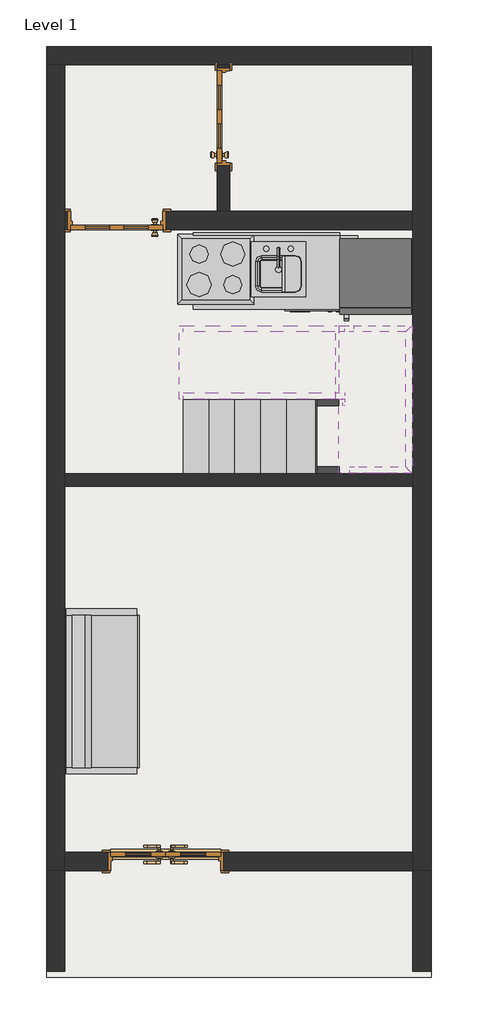
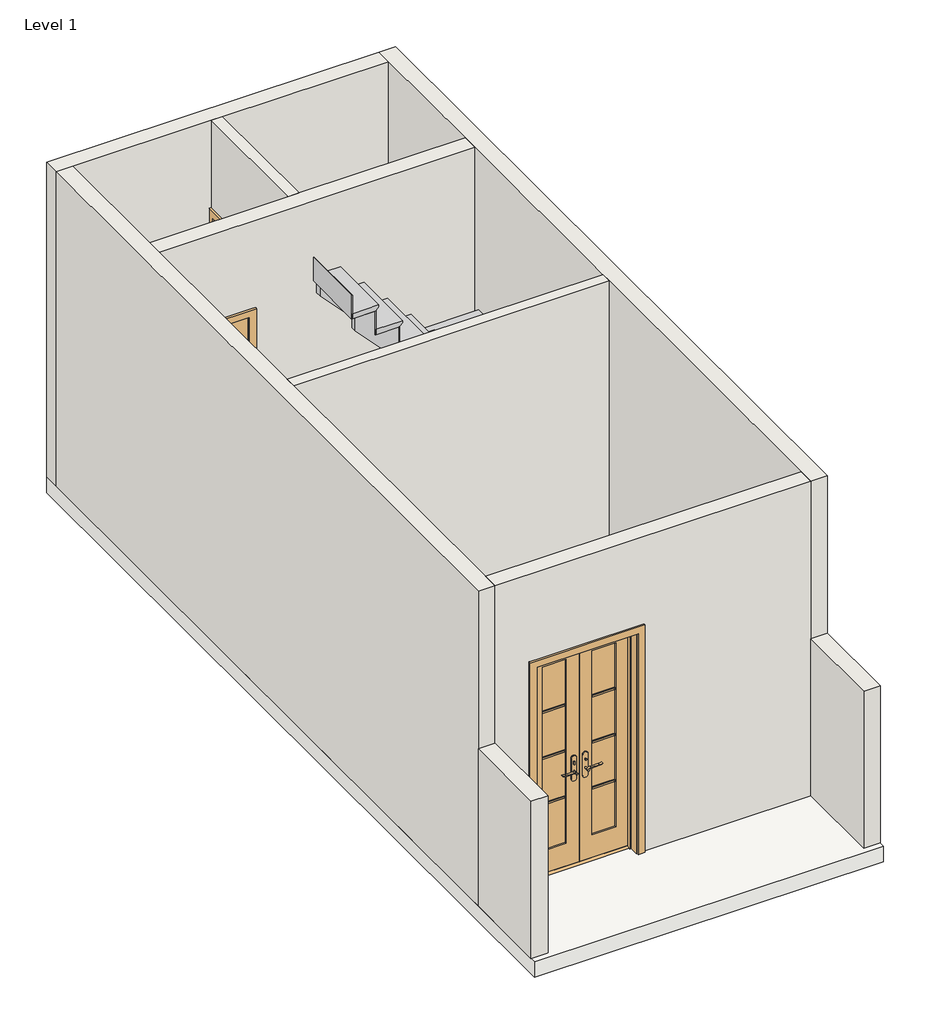
# One storey, incomplete: 9 walls, 8 members, 4 proxies, 3 doors, 2 furniture elements, 2 slabs, 2 stair flights, 1 flow terminal.
"""IFC4 building model written with IfcOpenShell, lengths in millimetres."""

from ifc_helpers import new_model, si_unit, frame, origin, origin_with_axes, place, context, project, spatial, polyline, outline, extrude, faceted_brep, transform, mapped, element, save
from components import proxy_a6faaae8, proxy_45b28599, kitchenette_medium_kitchenette_medium_5bfe328f, proxy_e2b28e2e, door_665efd91, door_a7370db0, door_bd7b73b2, flow_terminal_871c2e40, furniture_a1a13893, furniture_de36dbc2, non_monolithic_landing_e6237f85, stair_flight_15f1c366, stair_flight_6b27b35d

model = new_model("IFC4")

# Units and contexts
model_context = context("Model", 3, world=origin())
ifc_project = project(units=[si_unit("LENGTHUNIT", "METRE", prefix="MILLI")], contexts=[model_context])

# Site, building, storey
site = spatial("IfcSite", under=ifc_project)
building = spatial("IfcBuilding", under=site)
storey = spatial("IfcBuildingStorey", under=building, Name="Level 1", Elevation=0.0)

# Proxies
placement = place(None, origin())
proxy_shape = proxy_a6faaae8(model_context)
element("IfcBuildingElementProxy", 1, Name="Cook Top-4 Unit2 : 22\" x 20\"", ObjectType="Cook Top-4 Unit2 : 22\" x 20\"", at=placement, inside=storey, context=model_context, shape_type="MappedRepresentation", body=[
    mapped(proxy_shape, transform((-4318.156559, 5420.3980625, 0.0), x_axis=(1.0, 0.0, 0.0), y_axis=(0.0, 1.0, 0.0), z_axis=(0.0, 0.0, 1.0))),
])
proxy_2_shape = proxy_45b28599(model_context)
element("IfcBuildingElementProxy", 2, Name="Dishwasher : 24\" x 24\" x 34\"", ObjectType="Dishwasher : 24\" x 24\" x 34\"", at=placement, inside=storey, context=model_context, shape_type="MappedRepresentation", body=[
    mapped(proxy_2_shape, transform((-3824.1740275, 5128.5484977, 0.0), x_axis=(1.0, 0.0, 0.0), y_axis=(0.0, 1.0, 0.0), z_axis=(0.0, 0.0, 1.0))),
])
kitchenette_medium_kitchenette_medium_shape = kitchenette_medium_kitchenette_medium_5bfe328f(model_context)
element("IfcBuildingElementProxy", 3, Name="Kitchenette - Medium : Kitchenette - Medium", ObjectType="Kitchenette - Medium : Kitchenette - Medium", at=placement, inside=storey, context=model_context, shape_type="MappedRepresentation", body=[
    mapped(kitchenette_medium_kitchenette_medium_shape, transform((-4146.3942639, 5725.1980625, 0.0), x_axis=(1.0, 0.0, 0.0), y_axis=(0.0, 1.0, 0.0), z_axis=(0.0, 0.0, 1.0))),
])
proxy_3_shape = proxy_e2b28e2e(model_context)
element("IfcBuildingElementProxy", 4, Name="Refrigerator : 24\" x 25\" LH", ObjectType="Refrigerator : 24\" x 25\" LH", at=placement, inside=storey, context=model_context, shape_type="MappedRepresentation", body=[
    mapped(proxy_3_shape, transform((-2991.006559, 5374.749091, 0.0), x_axis=(1.0, 0.0, 0.0), y_axis=(0.0, 1.0, 0.0), z_axis=(0.0, 0.0, 1.0))),
])

# Doors
door_shape = door_665efd91(model_context)
element("IfcDoor", 5, ObjectType="Door-Exterior-Double-Full Glass-Wood_Clad : 36\" x 84\"", at=placement, inside=storey, context=model_context, shape_type="MappedRepresentation", body=[
    mapped(door_shape, transform((-4737.256559, 495.9730625, 0.0), x_axis=(1.0, 0.0, 0.0), y_axis=(0.0, 1.0, 0.0), z_axis=(0.0, 0.0, 1.0))),
])
door_2_shape = door_a7370db0(model_context)
element("IfcDoor", 6, ObjectType="Door-Interior-Single-4_Panel-Wood : 30\" x 84\"", at=placement, inside=storey, context=model_context, shape_type="MappedRepresentation", body=[
    mapped(door_2_shape, transform((-5143.656559, 5823.6230625, 0.0), x_axis=(-1.0, 0.0, 0.0), y_axis=(0.0, -1.0, 0.0), z_axis=(0.0, 0.0, 1.0))),
])
door_3_shape = door_bd7b73b2(model_context)
element("IfcDoor", 7, ObjectType="Door-Interior-Single-4_Panel-Wood : 30\" x 84\"", at=placement, inside=storey, context=model_context, shape_type="MappedRepresentation", body=[
    mapped(door_3_shape, transform((-4257.831559, 6690.3980625, 0.0), x_axis=(0.0, 1.0, 0.0), y_axis=(-1.0, 0.0, 0.0), z_axis=(0.0, 0.0, 1.0))),
])

# Flow terminal
flow_terminal_shape = flow_terminal_871c2e40(model_context)
element("IfcFlowTerminal", 8, ObjectType="Sink Kitchen-Island : 18\" x 18\"", at=placement, inside=storey, context=model_context, shape_type="MappedRepresentation", body=[
    mapped(flow_terminal_shape, transform((-3813.1457996, 5418.0526614, -14.4), x_axis=(1.0, 0.0, 0.0), y_axis=(0.0, 1.0, 0.0), z_axis=(0.0, 0.0, 1.0))),
])

# Furniture
furniture_shape = furniture_a1a13893(model_context)
element("IfcFurniture", 9, ObjectType="Counter Top w Sink Hole : 24\" Depth", at=placement, inside=storey, context=model_context, shape_type="MappedRepresentation", body=[
    mapped(furniture_shape, transform((-3308.1942639, 5725.1980625, -14.4), x_axis=(1.0, 0.0, 0.0), y_axis=(0.0, 1.0, 0.0), z_axis=(0.0, 0.0, 1.0))),
])
furniture_2_shape = furniture_de36dbc2(model_context)
element("IfcFurniture", 10, ObjectType="Sofa : 54\"", at=placement, inside=storey, context=model_context, shape_type="MappedRepresentation", body=[
    mapped(furniture_2_shape, transform((-5086.4024607, 1838.4775707, 0.0), x_axis=(0.0, 1.0000000000000002, 0.0), y_axis=(-1.0000000000000002, 0.0, 0.0), z_axis=(0.0, 0.0, 1.0))),
])

# Members
element("IfcMember", 11, ObjectType="Carriage - 2\" Width", at=placement, inside=storey, context=model_context, shape_type="Brep", body=[
    faceted_brep([(-3327.7737097, 4341.1083475, 1778.0), (-3327.7737097, 4391.9083475, 1778.0), (-3543.6737097, 4391.9083475, 1778.0), (-3543.6737097, 4341.1083475, 1778.0), (-3327.7737097, 4341.1083475, 1549.4), (-3327.7737097, 4391.9083475, 1549.4), (-3543.6737097, 4341.1083475, 2006.6), (-3543.6737097, 4391.9083475, 2006.6), (-3759.5737097, 4391.9083475, 2006.6), (-3759.5737097, 4341.1083475, 2006.6), (-3759.5737097, 4341.1083475, 2235.2), (-3759.5737097, 4391.9083475, 2235.2), (-3975.4737097, 4391.9083475, 2235.2), (-3975.4737097, 4341.1083475, 2235.2), (-3975.4737097, 4341.1083475, 2463.8), (-3975.4737097, 4391.9083475, 2463.8), (-4191.3737097, 4391.9083475, 2463.8), (-4191.3737097, 4341.1083475, 2463.8), (-4191.3737097, 4341.1083475, 2692.4), (-4191.3737097, 4391.9083475, 2692.4), (-4407.2737097, 4391.9083475, 2692.4), (-4407.2737097, 4341.1083475, 2692.4), (-4407.2737097, 4341.1083475, 2921.0), (-4407.2737097, 4391.9083475, 2921.0), (-4591.4237097, 4391.9083475, 2921.0), (-4591.4237097, 4341.1083475, 2921.0), (-3245.2237097, 4341.1083475, 1371.6), (-3245.2237097, 4391.9083475, 1371.6), (-3245.2237097, 4391.9083475, 1549.4), (-3245.2237097, 4341.1083475, 1549.4), (-3247.1951617, 4341.1083475, 1371.6), (-3247.1951617, 4391.9083475, 1371.6), (-4591.4237097, 4391.9083475, 2794.9008155), (-4591.4237097, 4341.1083475, 2794.9008155), (-3296.0237097, 4341.1083475, 1423.3008155), (-3327.7737097, 4341.1083475, 1456.9184625), (-3543.6737097, 4341.1083475, 1685.5184625), (-3759.5737097, 4341.1083475, 1914.1184625), (-3975.4737097, 4341.1083475, 2142.7184625), (-4191.3737097, 4341.1083475, 2371.3184625), (-4407.2737097, 4341.1083475, 2599.9184625), (-3296.0237097, 4341.1083475, 1549.4)], [[[0, 1, 2, 3]], [[1, 0, 4, 5]], [[6, 7, 8, 9]], [[3, 2, 7, 6]], [[10, 11, 12, 13]], [[9, 8, 11, 10]], [[14, 15, 16, 17]], [[13, 12, 15, 14]], [[18, 19, 20, 21]], [[17, 16, 19, 18]], [[22, 23, 24, 25]], [[21, 20, 23, 22]], [[26, 27, 28, 29]], [[26, 30, 31, 27]], [[32, 33, 25, 24]], [[31, 32, 24, 23, 20, 19, 16, 15, 12, 11, 8, 7, 2, 1, 5, 28, 27]], [[33, 32, 31, 30, 34, 35, 36, 37, 38, 39, 40]], [[30, 26, 29, 41, 4, 0, 3, 6, 9, 10, 13, 14, 17, 18, 21, 22, 25, 33, 40, 39, 38, 37, 36, 35, 34]], [[5, 4, 41, 29, 28]]]),
])
element("IfcMember", 12, ObjectType="Carriage - 2\" Width", at=placement, inside=storey, context=model_context, shape_type="Brep", body=[
    faceted_brep([(-4591.4237097, 4950.7083475, 2794.9008155), (-4591.4237097, 4899.9083475, 2794.9008155), (-4591.4237097, 4899.9083475, 2921.0), (-4591.4237097, 4950.7083475, 2921.0), (-3247.1951617, 4899.9083475, 1371.6), (-3170.555096, 4899.9083475, 1549.4), (-3327.7737097, 4899.9083475, 1549.4), (-3327.7737097, 4899.9083475, 1778.0), (-3543.6737097, 4899.9083475, 1778.0), (-3543.6737097, 4899.9083475, 2006.6), (-3759.5737097, 4899.9083475, 2006.6), (-3759.5737097, 4899.9083475, 2235.2), (-3975.4737097, 4899.9083475, 2235.2), (-3975.4737097, 4899.9083475, 2463.8), (-4191.3737097, 4899.9083475, 2463.8), (-4191.3737097, 4899.9083475, 2692.4), (-4407.2737097, 4899.9083475, 2692.4), (-4407.2737097, 4899.9083475, 2921.0), (-4407.2737097, 4950.7083475, 2599.9184625), (-4191.3737097, 4950.7083475, 2371.3184625), (-3975.4737097, 4950.7083475, 2142.7184625), (-3759.5737097, 4950.7083475, 1914.1184625), (-3543.6737097, 4950.7083475, 1685.5184625), (-3327.7737097, 4950.7083475, 1456.9184625), (-3296.0237097, 4950.7083475, 1423.3008155), (-3247.1951617, 4950.7083475, 1371.6), (-4407.2737097, 4950.7083475, 2921.0), (-4407.2737097, 4950.7083475, 2692.4), (-4191.3737097, 4950.7083475, 2692.4), (-4191.3737097, 4950.7083475, 2463.8), (-3975.4737097, 4950.7083475, 2463.8), (-3975.4737097, 4950.7083475, 2235.2), (-3759.5737097, 4950.7083475, 2235.2), (-3759.5737097, 4950.7083475, 2006.6), (-3543.6737097, 4950.7083475, 2006.6), (-3543.6737097, 4950.7083475, 1778.0), (-3327.7737097, 4950.7083475, 1778.0), (-3327.7737097, 4950.7083475, 1549.4), (-3296.0237097, 4950.7083475, 1549.4), (-3170.555096, 4950.7083475, 1549.4)], [[[0, 1, 2, 3]], [[1, 4, 5, 6, 7, 8, 9, 10, 11, 12, 13, 14, 15, 16, 17, 2]], [[1, 0, 18, 19, 20, 21, 22, 23, 24, 25, 4]], [[0, 3, 26, 27, 28, 29, 30, 31, 32, 33, 34, 35, 36, 37, 38, 39, 25, 24, 23, 22, 21, 20, 19, 18]], [[7, 36, 35, 8]], [[36, 7, 6, 37]], [[9, 34, 33, 10]], [[8, 35, 34, 9]], [[11, 32, 31, 12]], [[10, 33, 32, 11]], [[13, 30, 29, 14]], [[12, 31, 30, 13]], [[15, 28, 27, 16]], [[14, 29, 28, 15]], [[17, 26, 3, 2]], [[16, 27, 26, 17]], [[4, 25, 39, 5]], [[37, 6, 5, 39, 38]]]),
])
element("IfcMember", 13, ObjectType="Carriage - 2\" Width", at=placement, inside=storey, context=model_context, shape_type="Brep", body=[
    faceted_brep([(-4559.6737097, 4334.5480625, 0.0), (-4424.3522576, 4334.5480625, 0.0), (-4424.3522576, 4283.7480625, 0.0), (-4559.6737097, 4283.7480625, 0.0), (-3296.0237097, 4334.5480625, 1194.7008155), (-3296.0237097, 4283.7480625, 1194.7008155), (-4343.7737097, 4334.5480625, 85.3184625), (-4127.8737097, 4334.5480625, 313.9184625), (-3911.9737097, 4334.5480625, 542.5184625), (-3696.0737097, 4334.5480625, 771.1184625), (-3480.1737097, 4334.5480625, 999.7184625), (-3296.0237097, 4334.5480625, 1320.8), (-4559.6737097, 4334.5480625, 177.8), (-4343.7737097, 4334.5480625, 177.8), (-4343.7737097, 4334.5480625, 406.4), (-4127.8737097, 4334.5480625, 406.4), (-4127.8737097, 4334.5480625, 635.0), (-3911.9737097, 4334.5480625, 635.0), (-3911.9737097, 4334.5480625, 863.6), (-3696.0737097, 4334.5480625, 863.6), (-3696.0737097, 4334.5480625, 1092.2), (-3480.1737097, 4334.5480625, 1092.2), (-3480.1737097, 4334.5480625, 1320.8), (-3480.1737097, 4283.7480625, 1320.8), (-3296.0237097, 4283.7480625, 1320.8), (-3480.1737097, 4283.7480625, 1092.2), (-3696.0737097, 4283.7480625, 1092.2), (-3696.0737097, 4283.7480625, 863.6), (-3911.9737097, 4283.7480625, 863.6), (-3911.9737097, 4283.7480625, 635.0), (-4127.8737097, 4283.7480625, 635.0), (-4127.8737097, 4283.7480625, 406.4), (-4343.7737097, 4283.7480625, 406.4), (-4343.7737097, 4283.7480625, 177.8), (-4559.6737097, 4283.7480625, 177.8)], [[[0, 1, 2, 3]], [[4, 5, 2, 1, 6, 7, 8, 9, 10]], [[11, 4, 10, 9, 8, 7, 6, 1, 0, 12, 13, 14, 15, 16, 17, 18, 19, 20, 21, 22]], [[22, 23, 24, 11]], [[2, 5, 24, 23, 25, 26, 27, 28, 29, 30, 31, 32, 33, 34, 3]], [[34, 12, 0, 3]], [[12, 34, 33, 13]], [[13, 33, 32, 14]], [[14, 32, 31, 15]], [[15, 31, 30, 16]], [[16, 30, 29, 17]], [[17, 29, 28, 18]], [[18, 28, 27, 19]], [[19, 27, 26, 20]], [[20, 26, 25, 21]], [[21, 25, 23, 22]], [[5, 4, 11, 24]]]),
])
element("IfcMember", 14, ObjectType="Carriage - 2\" Width", at=placement, inside=storey, context=model_context, shape_type="Brep", body=[
    faceted_brep([(-4559.6737097, 3775.7480625, 0.0), (-4424.3522576, 3775.7480625, 0.0), (-4424.3522576, 3724.9480625, 0.0), (-4559.6737097, 3724.9480625, 0.0), (-3128.9522576, 3775.7480625, 1371.6), (-3128.9522576, 3724.9480625, 1371.6), (-3264.2737097, 3724.9480625, 1228.3184625), (-3296.0237097, 3724.9480625, 1194.7008155), (-3480.1737097, 3724.9480625, 999.7184625), (-3696.0737097, 3724.9480625, 771.1184625), (-3911.9737097, 3724.9480625, 542.5184625), (-4127.8737097, 3724.9480625, 313.9184625), (-4343.7737097, 3724.9480625, 85.3184625), (-3205.5923234, 3775.7480625, 1549.4), (-4559.6737097, 3775.7480625, 177.8), (-4343.7737097, 3775.7480625, 177.8), (-4343.7737097, 3775.7480625, 406.4), (-4127.8737097, 3775.7480625, 406.4), (-4127.8737097, 3775.7480625, 635.0), (-3911.9737097, 3775.7480625, 635.0), (-3911.9737097, 3775.7480625, 863.6), (-3696.0737097, 3775.7480625, 863.6), (-3696.0737097, 3775.7480625, 1092.2), (-3480.1737097, 3775.7480625, 1092.2), (-3480.1737097, 3775.7480625, 1320.8), (-3264.2737097, 3775.7480625, 1320.8), (-3264.2737097, 3775.7480625, 1549.4), (-3480.1737097, 3724.9480625, 1320.8), (-3296.0237097, 3724.9480625, 1320.8), (-3264.2737097, 3724.9480625, 1320.8), (-3205.5923234, 3724.9480625, 1549.4), (-3264.2737097, 3724.9480625, 1549.4), (-3480.1737097, 3724.9480625, 1092.2), (-3696.0737097, 3724.9480625, 1092.2), (-3696.0737097, 3724.9480625, 863.6), (-3911.9737097, 3724.9480625, 863.6), (-3911.9737097, 3724.9480625, 635.0), (-4127.8737097, 3724.9480625, 635.0), (-4127.8737097, 3724.9480625, 406.4), (-4343.7737097, 3724.9480625, 406.4), (-4343.7737097, 3724.9480625, 177.8), (-4559.6737097, 3724.9480625, 177.8)], [[[0, 1, 2, 3]], [[4, 5, 6, 7, 8, 9, 10, 11, 12, 2, 1]], [[13, 4, 1, 0, 14, 15, 16, 17, 18, 19, 20, 21, 22, 23, 24, 25, 26]], [[24, 27, 28, 29, 25]], [[5, 30, 31, 29, 28, 27, 32, 33, 34, 35, 36, 37, 38, 39, 40, 41, 3, 2, 12, 11, 10, 9, 8, 7, 6]], [[41, 14, 0, 3]], [[14, 41, 40, 15]], [[15, 40, 39, 16]], [[16, 39, 38, 17]], [[17, 38, 37, 18]], [[18, 37, 36, 19]], [[19, 36, 35, 20]], [[20, 35, 34, 21]], [[21, 34, 33, 22]], [[22, 33, 32, 23]], [[23, 32, 27, 24]], [[5, 4, 13, 30]], [[25, 29, 31, 26]], [[26, 31, 30, 13]]]),
])
element("IfcMember", 15, ObjectType="Carriage - 2\" Width", at=placement, inside=storey, context=model_context, shape_type="SweptSolid", body=[
    extrude(outline(polyline([(-3245.2237097, 4341.1083475), (-3245.2237097, 4283.7480625), (-3264.2737097, 4283.7480625), (-3264.2737097, 4334.5480625), (-3296.0237097, 4334.5480625), (-3296.0237097, 4341.1083475), (-3245.2237097, 4341.1083475)])), frame((0.0, 0.0, 1371.6), z_axis=(0.0, 0.0, 1.0), x_axis=(1.0, 0.0, 0.0)), (0.0, 0.0, 1.0), 177.8),
])
element("IfcMember", 16, ObjectType="Carriage - 2\" Width", at=placement, inside=storey, context=model_context, shape_type="Brep", body=[
    faceted_brep([(-2737.2237097, 3775.7480625, 1371.6), (-3128.9522576, 3775.7480625, 1371.6), (-3205.5923234, 3775.7480625, 1549.4), (-2737.2237097, 3775.7480625, 1549.4), (-2686.4237097, 3724.9480625, 1371.6), (-3128.9522576, 3724.9480625, 1371.6), (-2686.4237097, 3724.9480625, 1549.4), (-3205.5923234, 3724.9480625, 1549.4)], [[[0, 1, 2, 3]], [[1, 0, 4, 5]], [[5, 4, 6, 7]], [[3, 2, 7, 6]], [[1, 5, 7, 2]], [[4, 0, 3, 6]]]),
])
element("IfcMember", 17, ObjectType="Carriage - 2\" Width", at=placement, inside=storey, context=model_context, shape_type="SweptSolid", body=[
    extrude(outline(polyline([(-2737.2237097, 3775.7480625), (-2737.2237097, 4899.9083475), (-2686.4237097, 4950.7083475), (-2686.4237097, 3724.9480625), (-2737.2237097, 3775.7480625)])), frame((0.0, 0.0, 1371.6), z_axis=(0.0, 0.0, 1.0), x_axis=(1.0, 0.0, 0.0)), (0.0, 0.0, 1.0), 177.8),
])
element("IfcMember", 18, ObjectType="Carriage - 2\" Width", at=placement, inside=storey, context=model_context, shape_type="Brep", body=[
    faceted_brep([(-3247.1951617, 4899.9083475, 1371.6), (-2737.2237097, 4899.9083475, 1371.6), (-2737.2237097, 4899.9083475, 1549.4), (-3170.555096, 4899.9083475, 1549.4), (-3247.1951617, 4950.7083475, 1371.6), (-2686.4237097, 4950.7083475, 1371.6), (-3170.555096, 4950.7083475, 1549.4), (-2686.4237097, 4950.7083475, 1549.4)], [[[0, 1, 2, 3]], [[1, 0, 4, 5]], [[5, 4, 6, 7]], [[3, 2, 7, 6]], [[1, 5, 7, 2]], [[4, 0, 3, 6]]]),
])

# Slabs
element("IfcSlab", 19, ObjectType="6\"", at=placement, inside=storey, context=model_context, shape_type="SweptSolid", body=[
    extrude(outline(polyline([(-2527.456559, 7274.5980625), (-2527.456559, -472.4019375), (-5727.856559, -472.4019375), (-5727.856559, 7274.5980625), (-2527.456559, 7274.5980625)])), frame((0.0, 0.0, -152.4), z_axis=(0.0, 0.0, 1.0), x_axis=(1.0, 0.0, 0.0)), (0.0, 0.0, 1.0), 152.4),
])
non_monolithic_landing_shape = non_monolithic_landing_e6237f85(model_context)
element("IfcSlab", 20, ObjectType="Non-Monolithic Landing", at=placement, inside=storey, context=model_context, shape_type="MappedRepresentation", body=[
    mapped(non_monolithic_landing_shape, transform((0.0, 0.0, 0.0), x_axis=(1.0, 0.0, 0.0), y_axis=(0.0, 1.0, 0.0), z_axis=(0.0, 0.0, 1.0))),
])

# Stair flights
stair_flight_shape = stair_flight_15f1c366(model_context)
element("IfcStairFlight", 21, ObjectType="2\" Tread 1\" Nosing 1/4\" Riser", at=placement, inside=storey, context=model_context, shape_type="MappedRepresentation", body=[
    mapped(stair_flight_shape, transform((0.0, 0.0, 0.0), x_axis=(1.0, 0.0, 0.0), y_axis=(0.0, 1.0, 0.0), z_axis=(0.0, 0.0, 1.0))),
])
stair_flight_2_shape = stair_flight_6b27b35d(model_context)
element("IfcStairFlight", 22, ObjectType="2\" Tread 1\" Nosing 1/4\" Riser", at=placement, inside=storey, context=model_context, shape_type="MappedRepresentation", body=[
    mapped(stair_flight_2_shape, transform((0.0, 0.0, 0.0), x_axis=(1.0, 0.0, 0.0), y_axis=(0.0, 1.0, 0.0), z_axis=(0.0, 0.0, 1.0))),
])

# Walls
element("IfcWall", 23, ObjectType="4\"", at=placement, inside=storey, context=model_context, shape_type="SweptSolid", body=[
    extrude(outline(polyline([(5902.9980625, 3048.0), (7122.1980625, 3048.0), (7122.1980625, 0.0), (7096.7980625, 0.0), (7096.7980625, 2159.0), (6283.9980625, 2159.0), (6283.9980625, 0.0), (5902.9980625, 0.0), (5902.9980625, 3048.0)])), frame((-4305.456559, 0.0, 0.0), z_axis=(1.0, 0.0, 0.0), x_axis=(0.0, 1.0, 0.0)), (0.0, 0.0, 1.0), 101.6),
])
element("IfcWall", 24, ObjectType="4\"", at=placement, inside=storey, context=model_context, shape_type="SweptSolid", body=[
    extrude(outline(polyline([(-5575.456559, 3718.5980625), (-2679.856559, 3718.5980625), (-2679.856559, 3616.9980625), (-5575.456559, 3616.9980625), (-5575.456559, 3718.5980625)])), origin_with_axes(), (0.0, 0.0, 1.0), 3048.0),
])
element("IfcWall", 25, ObjectType="6\"", at=placement, inside=storey, context=model_context, shape_type="Brep", body=[
    faceted_brep([(-5727.856559, 7122.1980625, 0.0), (-5575.456559, 7122.1980625, 0.0), (-4305.456559, 7122.1980625, 0.0), (-4203.856559, 7122.1980625, 0.0), (-2679.856559, 7122.1980625, 0.0), (-2679.856559, 7122.1980625, 3048.0), (-4203.856559, 7122.1980625, 3048.0), (-4305.456559, 7122.1980625, 3048.0), (-5575.456559, 7122.1980625, 3048.0), (-5727.856559, 7122.1980625, 3048.0), (-5727.856559, 7274.5980625, 0.0), (-5727.856559, 7274.5980625, 3048.0), (-2679.856559, 7274.5980625, 3048.0), (-2679.856559, 7274.5980625, 0.0)], [[[0, 1, 2, 3, 4, 5, 6, 7, 8, 9]], [[10, 11, 12, 13]], [[4, 3, 2, 1, 0, 10, 13]], [[9, 8, 7, 6, 5, 12, 11]], [[0, 9, 11, 10]], [[5, 4, 13, 12]]]),
])
element("IfcWall", 26, ObjectType="6\"", at=placement, inside=storey, context=model_context, shape_type="SweptSolid", body=[
    extrude(outline(polyline([(-5575.456559, 416.5980625), (-5575.456559, -421.6019375), (-5727.856559, -421.6019375), (-5727.856559, 416.5980625), (-5575.456559, 416.5980625)])), origin_with_axes(), (0.0, 0.0, 1.0), 1524.0),
])
element("IfcWall", 27, ObjectType="6\"", at=placement, inside=storey, context=model_context, shape_type="Brep", body=[
    faceted_brep([(-2679.856559, 7274.5980625, 0.0), (-2679.856559, 7122.1980625, 0.0), (-2679.856559, 5902.9980625, 0.0), (-2679.856559, 5750.5980625, 0.0), (-2679.856559, 3718.5980625, 0.0), (-2679.856559, 3616.9980625, 0.0), (-2679.856559, 568.9980625, 0.0), (-2679.856559, 416.5980625, 0.0), (-2679.856559, 416.5980625, 1524.0), (-2679.856559, 416.5980625, 3048.0), (-2679.856559, 568.9980625, 3048.0), (-2679.856559, 3616.9980625, 3048.0), (-2679.856559, 3718.5980625, 3048.0), (-2679.856559, 5750.5980625, 3048.0), (-2679.856559, 5902.9980625, 3048.0), (-2679.856559, 7122.1980625, 3048.0), (-2679.856559, 7274.5980625, 3048.0), (-2527.456559, 7274.5980625, 0.0), (-2527.456559, 7274.5980625, 3048.0), (-2527.456559, 416.5980625, 3048.0), (-2527.456559, 416.5980625, 1524.0), (-2527.456559, 416.5980625, 0.0)], [[[0, 1, 2, 3, 4, 5, 6, 7, 8, 9, 10, 11, 12, 13, 14, 15, 16]], [[17, 18, 19, 20, 21]], [[7, 6, 5, 4, 3, 2, 1, 0, 17, 21]], [[9, 8, 7, 21, 20, 19]], [[16, 15, 14, 13, 12, 11, 10, 9, 19, 18]], [[0, 16, 18, 17]]]),
])
element("IfcWall", 28, ObjectType="6\"", at=placement, inside=storey, context=model_context, shape_type="SweptSolid", body=[
    extrude(outline(polyline([(3048.0, -2679.856559), (3048.0, -5575.456559), (0.0, -5575.456559), (0.0, -5219.856559), (2159.0, -5219.856559), (2159.0, -4254.656559), (0.0, -4254.656559), (0.0, -2679.856559), (3048.0, -2679.856559)])), frame((0.0, 416.5980625, 0.0), z_axis=(0.0, 1.0, 0.0), x_axis=(0.0, 0.0, 1.0)), (0.0, 0.0, 1.0), 152.4),
])
element("IfcWall", 29, ObjectType="6\"", at=placement, inside=storey, context=model_context, shape_type="Brep", body=[
    faceted_brep([(-2679.856559, 5750.5980625, 3048.0), (-5575.456559, 5750.5980625, 3048.0), (-5575.456559, 5750.5980625, 0.0), (-5550.056559, 5750.5980625, 0.0), (-5550.056559, 5750.5980625, 2159.0), (-4737.256559, 5750.5980625, 2159.0), (-4737.256559, 5750.5980625, 0.0), (-2679.856559, 5750.5980625, 0.0), (-5575.456559, 5902.9980625, 3048.0), (-4305.456559, 5902.9980625, 3048.0), (-4203.856559, 5902.9980625, 3048.0), (-2679.856559, 5902.9980625, 3048.0), (-2679.856559, 5902.9980625, 0.0), (-4203.856559, 5902.9980625, 0.0), (-4305.456559, 5902.9980625, 0.0), (-4737.256559, 5902.9980625, 0.0), (-4737.256559, 5902.9980625, 2159.0), (-5550.056559, 5902.9980625, 2159.0), (-5550.056559, 5902.9980625, 0.0), (-5575.456559, 5902.9980625, 0.0)], [[[0, 1, 2, 3, 4, 5, 6, 7]], [[8, 9, 10, 11, 12, 13, 14, 15, 16, 17, 18, 19]], [[2, 19, 18, 3]], [[12, 7, 6, 15, 14, 13]], [[1, 0, 11, 10, 9, 8]], [[2, 1, 8, 19]], [[0, 7, 12, 11]], [[17, 4, 3, 18]], [[4, 17, 16, 5]], [[5, 16, 15, 6]]]),
])
element("IfcWall", 30, ObjectType="6\"", at=placement, inside=storey, context=model_context, shape_type="SweptSolid", body=[
    extrude(outline(polyline([(-2679.856559, -421.6019375), (-2679.856559, 416.5980625), (-2527.456559, 416.5980625), (-2527.456559, -421.6019375), (-2679.856559, -421.6019375)])), origin_with_axes(), (0.0, 0.0, 1.0), 1524.0),
])
element("IfcWall", 31, ObjectType="6\"", at=placement, inside=storey, context=model_context, shape_type="Brep", body=[
    faceted_brep([(-5575.456559, 416.5980625, 0.0), (-5575.456559, 568.9980625, 0.0), (-5575.456559, 3616.9980625, 0.0), (-5575.456559, 3718.5980625, 0.0), (-5575.456559, 5750.5980625, 0.0), (-5575.456559, 5902.9980625, 0.0), (-5575.456559, 7122.1980625, 0.0), (-5575.456559, 7122.1980625, 3048.0), (-5575.456559, 5902.9980625, 3048.0), (-5575.456559, 5750.5980625, 3048.0), (-5575.456559, 3718.5980625, 3048.0), (-5575.456559, 3616.9980625, 3048.0), (-5575.456559, 568.9980625, 3048.0), (-5575.456559, 416.5980625, 3048.0), (-5575.456559, 416.5980625, 1524.0), (-5727.856559, 416.5980625, 0.0), (-5727.856559, 416.5980625, 1524.0), (-5727.856559, 416.5980625, 3048.0), (-5727.856559, 7122.1980625, 3048.0), (-5727.856559, 7122.1980625, 0.0)], [[[0, 1, 2, 3, 4, 5, 6, 7, 8, 9, 10, 11, 12, 13, 14]], [[15, 16, 17, 18, 19]], [[6, 5, 4, 3, 2, 1, 0, 15, 19]], [[13, 12, 11, 10, 9, 8, 7, 18, 17]], [[0, 14, 13, 17, 16, 15]], [[7, 6, 19, 18]]]),
])

save(model, "model.ifc")

# Revit data of these elements
# Type "Cook Top-4 Unit2 : 22\" x 20\""
#   Depth = 1' - 8"
#   Width = 1' - 10"
#   Burner Material = Steel, Chrome Plated
#   Cooktop Material = Steel, Polished
#   Default Elevation = 0
#   Assembly Code = ""
# Type "Dishwasher : 24\" x 24\" x 34\""
#   Label = "DW"
#   Assembly Code = "E1090400"
#   Depth = 2' - 0"
#   Height = 2' - 10"
#   Width = 2' - 0"
#   Dishwasher Material = Steel, Paint Finish, Ivory, Glossy
#   Panel Face Material = Plastic, Opaque Black
#   Default Elevation = 0
# Type "Kitchenette - Medium : Kitchenette - Medium"
#   Assembly Code = "E1090400"
#   Counter Length = 4' - 0"
#   Cabinet Width = 2' - 6"
#   Cabinet Height = 2' - 10 1/2"
#   Cabinet Depth = 2' - 0"
#   Toe Depth = 0' - 3"
#   Toe Height = 0' - 3 1/2"
#   Cabinet Material = Cabinets
#   Door/Drawer Material = Cabinets
#   Handle Material = Cabinets - Handles
#   Default Elevation = 0
# Type "Refrigerator : 24\" x 25\" LH"
#   Label = "REF."
#   Assembly Code = "E1090400"
#   Depth = 2' - 0 3/4"
#   Handle = 0' - 1 1/2"
#   Height = 5' - 0"
#   Rear Clearance = 0' - 2"
#   Top Door Height = 1' - 8"
#   Width = 1' - 11 1/2"
#   Material = Steel, Paint Finish, Ivory, Glossy
#   Default Elevation = 0
# Type "Door-Exterior-Double-Full Glass-Wood_Clad : 36\" x 84\""
#   Type Mark = "10"
#   Assembly Code = "B2030100"
#   Analytic Construction = "French door, wood frame with double glass"
#   Top Rail = 0' - 4 11/16"
#   Threshold Offset [instance default] = 0' - 0 1/2"
#   Thickness = 0' - 1 3/8"
#   Thermal Resistance (R) = 1.9158 (h·ft²·°F)/BTU
#   Swing Angle [instance default] = 90.00°
#   Stiles = 0' - 4 3/4"
#   Rough Width = 3' - 2"
#   Rough Height = 7' - 1"
#   Panel Width = 1' - 6"
#   Door Offset [instance default] = 0' - 0"
#   Height = 7' - 0"
#   Width = 3' - 0"
#   Heat Transfer Coefficient (U) = 0.5220 BTU/(h·ft²·°F)
#   Bottom Rail = 0' - 9 1/8"
#   Exterior Trim [instance default] = yes
#   Threshold [instance default] = yes
#   Show Grill [instance default] = yes
#   Function = 1
#   Trim Material = Cherry
#   Threshold Material = Cherry
#   Panel Material = Cherry
#   Glazing = Glass
#   Frame Material = Cherry
#   Door Handle Material = Aluminum
#   Visual Light Transmittance = 0
#   Solar Heat Gain Coefficient = 0
#   Wall Closure = (empty or 0)
#   Construction Type = (empty or 0)
# Type "Door-Interior-Single-4_Panel-Wood : 30\" x 84\""
#   Type Mark = "9"
#   Assembly Code = "C1020300"
#   Analytic Construction = "Wooden"
#   Top Rail = 0' - 4 11/16"
#   Thickness = 0' - 1 3/8"
#   Thermal Resistance (R) = 2.5876 (h·ft²·°F)/BTU
#   Swing Angle [instance default] = 90.00°
#   Stiles = 0' - 4 3/4"
#   Rough Width = 2' - 8"
#   Rough Height = 7' - 1"
#   Mullion = 0' - 4 1/2"
#   Lock Rail = 0' - 7 1/2"
#   Height = 7' - 0"
#   Width = 2' - 6"
#   Heat Transfer Coefficient (U) = 0.3865 BTU/(h·ft²·°F)
#   Bottom Rail = 0' - 9 1/8"
#   Trim Material = Cherry
#   Panel Material = Cherry
#   Frame Material = Cherry
#   Door Handle Material = Aluminum
#   Visual Light Transmittance = 0
#   Solar Heat Gain Coefficient = 0
#   Wall Closure = (empty or 0)
#   Function = (empty or 0)
# Type "Sink Kitchen-Island : 18\" x 18\""
#   Assembly Code = "D2010410"
#   Counter Height = 3' - 0"
#   Depth = 1' - 6"
#   Width = 1' - 6"
#   Faucet Material = Steel, Polished
#   Sink Material = Steel, Polished
#   Default Elevation = 0
# Type "Counter Top w Sink Hole : 24\" Depth"
#   Assembly Code = "C1030400"
#   Counter Thickness = 0' - 1 1/2"
#   Depth [instance default] = 2' - 1"
#   Height = 3' - 0"
#   Length [instance default] = 8' - 0"
#   Sink Location [instance default] = 2' - 0"
#   Sink Location To Wall [instance default] = 0' - 6"
#   Sink Opening Depth [instance default] = 1' - 3"
#   Sink Opening Width [instance default] = 2' - 3"
#   Counter Top Material = none
#   Default Elevation = 0
# Type "Sofa : 54\""
#   Assembly Code = "E2020200"
#   Width = 4' - 6"
#   Seat Material = none
#   Frame Material = none
#   Default Elevation = 0
# Type "6\""
#   Assembly Code = "B1010"
#   Function = 0
#   Layers, outside or top first: 0' - 6" no material (function 1)
# Type "4\""
#   Assembly Code = "B2010"
#   Layers, outside or top first: 0' - 4" no material (function 1)
# Type "6\""
#   Assembly Code = "B2010"
#   Layers, outside or top first: 0' - 6" "ext wall" (function 1)
# Element 1 (IfcBuildingElementProxy, "Cook Top-4 Unit2 : 22\" x 20\"")
#   Phase Created = New Construction
#   Materials on its faces: "Steel, Chrome Plated", "Steel, Polished"
# Element 2 (IfcBuildingElementProxy, "Dishwasher : 24\" x 24\" x 34\"")
#   Phase Created = New Construction
#   Materials on its faces: "Steel, Paint Finish, Ivory, Glossy", "Plastic, Opaque Black"
# Element 3 (IfcBuildingElementProxy, "Kitchenette - Medium : Kitchenette - Medium")
#   Phase Created = New Construction
#   Materials on its faces: "Cabinets", "Cabinets - Handles"
# Element 4 (IfcBuildingElementProxy, "Refrigerator : 24\" x 25\" LH")
#   Phase Created = New Construction
#   Materials on its faces: "Steel, Paint Finish, Ivory, Glossy", "Steel, Chrome Plated"
# Element 5 (IfcDoor, "Door-Exterior-Double-Full Glass-Wood_Clad : 36\" x 84\"")
#   Threshold Offset = 0' - 0 1/2"
#   Swing Angle = 90.00°
#   Door Offset = 0' - 0"
#   Threshold = yes
#   Show Grill = yes
#   Exterior Trim = yes
#   Phase Created = New Construction
#   Materials on its faces: "Cherry", "Aluminum", "Glass"
# Elements 6, 7 (IfcDoor, "Door-Interior-Single-4_Panel-Wood : 30\" x 84\"")
#   Swing Angle = 90.00°
#   Phase Created = New Construction
#   Materials on its faces: "Cherry", "Aluminum"
# Element 8 (IfcFlowTerminal, "Sink Kitchen-Island : 18\" x 18\"")
#   Mark = "4"
#   Phase Created = New Construction
#   Materials on its faces: "Steel, Polished"
# Element 9 (IfcFurniture, "Counter Top w Sink Hole : 24\" Depth")
#   Sink Opening Depth = 1' - 2"
#   Sink Location To Wall = 0' - 6"
#   Length = 4' - 0"
#   Sink Location = 2' - 4"
#   Sink Opening Width = 1' - 4"
#   Depth = 2' - 1"
#   Phase Created = New Construction
#   Materials on its faces: "Counter Top"
# Element 10 (IfcFurniture, "Sofa : 54\"")
#   Phase Created = New Construction
#   Materials on its faces: "Cherry"
# Elements 11, 12, 13, 14, 15, 16, 17, 18 (IfcMember, "Carriage - 2\" Width")
#   Phase Created = New Construction
# Element 19 (IfcSlab, "6\"")
#   Height Offset From Level = 0' - 0"
#   Phase Created = New Construction
#   Materials on its faces: "Default Floor"
# Element 20 (IfcSlab, "Non-Monolithic Landing")
#   Phase Created = New Construction
# Elements 21, 22 (IfcStairFlight, "2\" Tread 1\" Nosing 1/4\" Riser")
#   Phase Created = New Construction
# Elements 23, 24 (IfcWall, "4\"")
#   Top Offset = 0' - 0"
#   Base Offset = 0' - 0"
#   Unconnected Height = 10' - 0"
#   wall height = 10' - 0"
#   Phase Created = New Construction
#   Base Constraint = Level 1
#   Materials on its faces: "Default Wall"
# Elements 25, 27, 28, 29, 31 (IfcWall, "6\"")
#   Top Offset = 0' - 0"
#   Base Offset = 0' - 0"
#   Unconnected Height = 10' - 0"
#   wall height = 10' - 0"
#   Phase Created = New Construction
#   Base Constraint = Level 1
#   Materials on its faces: "ext wall"
# Elements 26, 30 (IfcWall, "6\"")
#   Top Offset = 0' - 0"
#   Base Offset = 0' - 0"
#   Unconnected Height = 5' - 0"
#   wall height = 5' - 0"
#   Phase Created = New Construction
#   Base Constraint = Level 1
#   Materials on its faces: "ext wall"
# Materials
#   "Steel, Chrome Plated": class "Metal", colour RGB 17 17 17, transparency 0, Description = "Chromiuim plated steel", Cost = 0
#   "Steel, Polished": class "Metal", colour RGB 57 57 57, transparency 0, Description = "Polished steel", Cost = 0
#   "Steel, Paint Finish, Ivory, Glossy": class "Metal", colour RGB 247 247 239, transparency 0, Description = "Steel, paint finish, ivory, glossy", Cost = 0
#   "Plastic, Opaque Black": class "Plastic", colour RGB 0 0 0, transparency 0.7, Description = "Plastic, generic, opaque black", Cost = 0
#   "Cabinets": colour RGB 249 249 249, transparency 0
#   "Cabinets - Handles": class "Metal", colour RGB 57 57 57, transparency 0
#   "Cherry": class "Wood", colour RGB 226 177 128, transparency 0, Description = "Prunus Serotina", Cost = 0
#   "Glass": class "Glass", colour RGB 0 128 192, transparency 0.75, Description = "Soda Lime Glass", Cost = 0
#   "Aluminum": class "Metal", colour RGB 247 247 247, transparency 0, Description = "Aluminum 6061", Cost = 0
#   "ext wall": class "Generic", colour RGB 187 179 160, transparency 0, Cost = 0
#   "Counter Top": class "Wood", colour RGB 226 177 128, transparency 0
#   "Default Floor": colour RGB 128 128 128, transparency 0
#   "Default Wall": colour RGB 128 128 128, transparency 0
